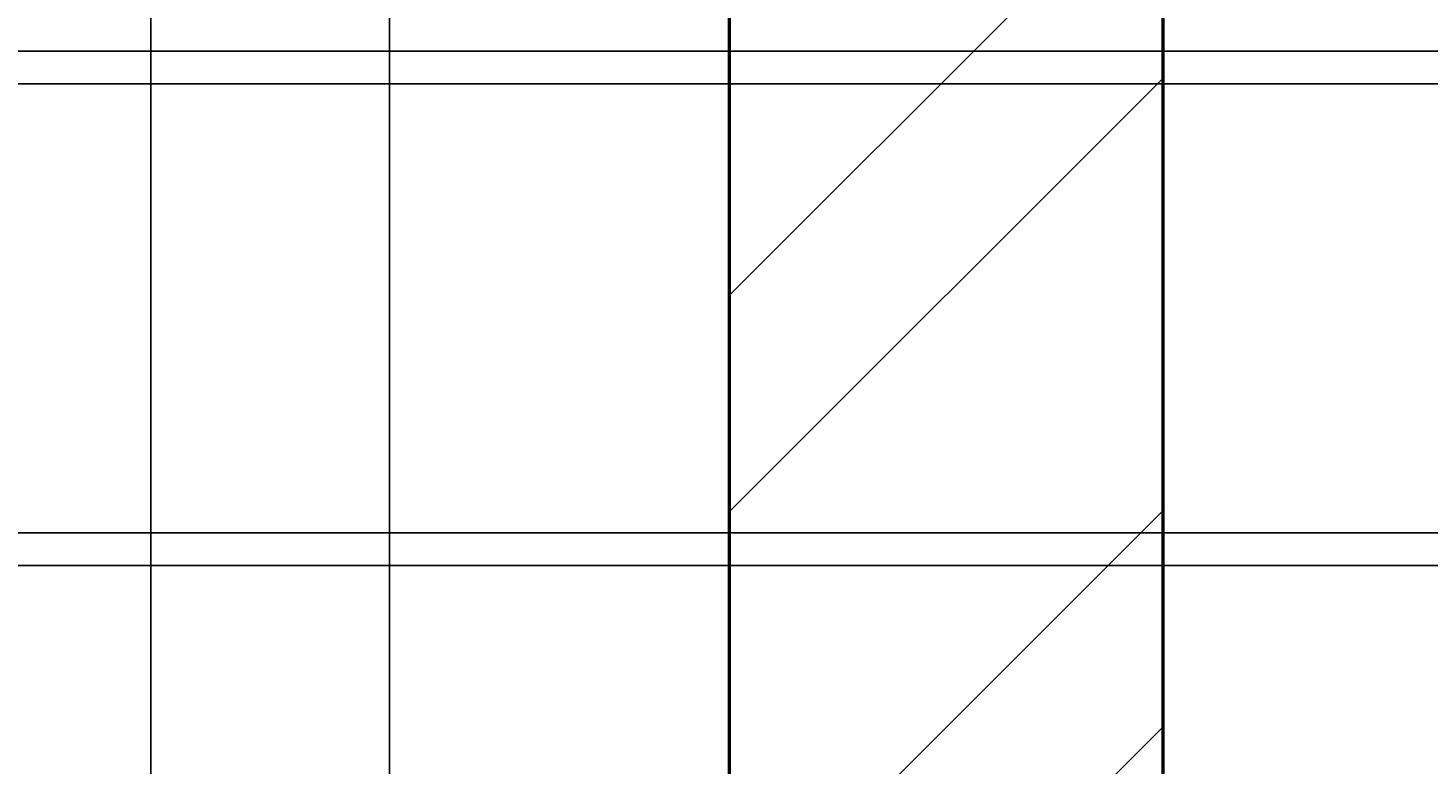
# Model space of a CAD drawing. Units: inches. Extents: x 2812 to 3051, y 1398 to 1659.
# Tile 35 of 65: x 3004 to 3033, y 1433 to 1448. Entities that reach past the tile are written whole.
import ezdxf

# ---------------------------------------------------------------- set-up
doc = ezdxf.new("R2010")
doc.units = ezdxf.units.IN
for name, color, linetype, lineweight in [('A-ANNO-DIMS', 2, 'Continuous', 18), ('S-CONC', 7, 'Continuous', 50), ('S-CONC-PATT', 8, 'Continuous', 18)]:
    doc.layers.add(name, color=color, linetype=linetype, lineweight=lineweight)
doc.styles.get("Standard").update_dxf_attribs({"font": 'arial.ttf'})
doc.dimstyles.get("Standard").update_dxf_attribs({"dimtxt": 0.18, "dimasz": 0.18, "dimexe": 0.18, "dimexo": 0.0625, "dimgap": 0.09, "dimtad": 0, "dimtih": 1, "dimtoh": 1, "dimdec": 4, "dimzin": 0, "dimdsep": 46, "dimtxsty": 'Standard', "dimcen": 0.09, "dimadec": 0, "dimazin": 0, "dimtfac": 1, "dimtdec": 4, "dimtofl": 0, "dimtmove": 0, "dimatfit": 3, "dimfxl": 1, "dimtolj": 1, "dimtzin": 0, "dimarcsym": 0})

# ---------------------------------------------------------------- blocks, each defined once
blk = doc.blocks.new('*D33')
at = {"layer": 'A-ANNO-DIMS', "color": 0, "lineweight": -2, "transparency": 16777216}
for p, q in [((3011.337, 1597.982), (3011.337, 1397.505)), ((3018.385, 1559.757), (3018.385, 1397.505)), ((3011.517, 1397.685), (3014.468, 1397.685)), ((3018.205, 1397.685), (3015.254, 1397.685))]:
    blk.add_line(p, q, dxfattribs=at)
at = {"layer": 'A-ANNO-DIMS', "color": 0, "transparency": 16777216}
for points in [[(3011.517, 1397.715), (3011.517, 1397.655), (3011.337, 1397.685)], [(3018.205, 1397.715), (3018.205, 1397.655), (3018.385, 1397.685)]]:
    blk.add_solid(points, dxfattribs=at)
at = {"layer": 'Defpoints', "color": 0, "transparency": 16777216}
for p in [(3011.337, 1598.044), (3018.385, 1559.82), (3018.385, 1397.685)]:
    blk.add_point(p, dxfattribs=at)
at = {"layer": 'A-ANNO-DIMS', "color": 0, "transparency": 16777216, "insert": (3014.861, 1397.685), "char_height": 0.18, "attachment_point": 5}
blk.add_mtext('\\A1;7.048', dxfattribs=at)
blk = doc.blocks.new('*D34')
at = {"layer": 'A-ANNO-DIMS', "color": 0, "lineweight": -2, "transparency": 16777216}
for p, q in [((3038.462, 1593.482), (3038.462, 1397.505)), ((3027.385, 1550.757), (3027.385, 1397.505)), ((3027.565, 1397.685), (3032.468, 1397.685)), ((3038.282, 1397.685), (3033.379, 1397.685))]:
    blk.add_line(p, q, dxfattribs=at)
at = {"layer": 'A-ANNO-DIMS', "color": 0, "transparency": 16777216}
for points in [[(3027.565, 1397.715), (3027.565, 1397.655), (3027.385, 1397.685)], [(3038.282, 1397.715), (3038.282, 1397.655), (3038.462, 1397.685)]]:
    blk.add_solid(points, dxfattribs=at)
at = {"layer": 'Defpoints', "color": 0, "transparency": 16777216}
for p in [(3038.462, 1593.544), (3027.385, 1550.82), (3038.462, 1397.685)]:
    blk.add_point(p, dxfattribs=at)
at = {"layer": 'A-ANNO-DIMS', "color": 0, "transparency": 16777216, "insert": (3032.923, 1397.685), "char_height": 0.18, "attachment_point": 5}
blk.add_mtext('\\A1;11.077', dxfattribs=at)
blk = doc.blocks.new('*D47')
at = {"layer": 'A-ANNO-DIMS', "color": 0, "lineweight": -2, "transparency": 16777216}
for p, q in [((2970.385, 1487.973), (2970.385, 1397.505)), ((3006.385, 1487.973), (3006.385, 1397.505)), ((2970.565, 1397.685), (2988.166, 1397.685)), ((3006.205, 1397.685), (2988.604, 1397.685))]:
    blk.add_line(p, q, dxfattribs=at)
at = {"layer": 'A-ANNO-DIMS', "color": 0, "transparency": 16777216}
for points in [[(2970.565, 1397.715), (2970.565, 1397.655), (2970.385, 1397.685)], [(3006.205, 1397.715), (3006.205, 1397.655), (3006.385, 1397.685)]]:
    blk.add_solid(points, dxfattribs=at)
at = {"layer": 'Defpoints', "color": 0, "transparency": 16777216}
for p in [(2970.385, 1488.035), (3006.385, 1488.035), (3006.385, 1397.685)]:
    blk.add_point(p, dxfattribs=at)
at = {"layer": 'A-ANNO-DIMS', "color": 0, "transparency": 16777216, "insert": (2988.385, 1397.685), "char_height": 0.18, "attachment_point": 5}
blk.add_mtext('\\A1;36', dxfattribs=at)
blk = doc.blocks.new('*D48')
at = {"layer": 'A-ANNO-DIMS', "color": 0, "lineweight": -2, "transparency": 16777216}
for p, q in [((3006.385, 1487.973), (3006.385, 1397.505)), ((3036.385, 1409.973), (3036.385, 1397.505)), ((3006.565, 1397.685), (3021.166, 1397.685)), ((3036.205, 1397.685), (3021.603, 1397.685))]:
    blk.add_line(p, q, dxfattribs=at)
at = {"layer": 'A-ANNO-DIMS', "color": 0, "transparency": 16777216}
for points in [[(3006.565, 1397.715), (3006.565, 1397.655), (3006.385, 1397.685)], [(3036.205, 1397.715), (3036.205, 1397.655), (3036.385, 1397.685)]]:
    blk.add_solid(points, dxfattribs=at)
at = {"layer": 'Defpoints', "color": 0, "transparency": 16777216}
for p in [(3006.385, 1488.035), (3036.385, 1410.035), (3036.385, 1397.685)]:
    blk.add_point(p, dxfattribs=at)
at = {"layer": 'A-ANNO-DIMS', "color": 0, "transparency": 16777216, "insert": (3021.385, 1397.685), "char_height": 0.18, "attachment_point": 5}
blk.add_mtext('\\A1;30', dxfattribs=at)
blk = doc.blocks.new('*D65')
at = {"layer": 'A-ANNO-DIMS', "color": 0, "lineweight": -2, "transparency": 16777216}
for p, q in [((2920.62, 1437.426), (3051.178, 1437.426)), ((3050.998, 1437.246), (3050.998, 1432.608)), ((3050.998, 1427.606), (3050.998, 1432.245)), ((2929.438, 1427.426), (3051.178, 1427.426))]:
    blk.add_line(p, q, dxfattribs=at)
at = {"layer": 'A-ANNO-DIMS', "color": 0, "transparency": 16777216}
for points in [[(3050.968, 1437.246), (3051.028, 1437.246), (3050.998, 1437.426)], [(3050.968, 1427.606), (3051.028, 1427.606), (3050.998, 1427.426)]]:
    blk.add_solid(points, dxfattribs=at)
at = {"layer": 'Defpoints', "color": 0, "transparency": 16777216}
for p in [(2920.558, 1437.426), (3050.998, 1437.426), (2929.375, 1427.426)]:
    blk.add_point(p, dxfattribs=at)
at = {"layer": 'A-ANNO-DIMS', "color": 0, "transparency": 16777216, "insert": (3050.998, 1432.426), "char_height": 0.18, "attachment_point": 5}
blk.add_mtext('\\A1;10', dxfattribs=at)
blk = doc.blocks.new('*D66')
at = {"layer": 'A-ANNO-DIMS', "color": 0, "lineweight": -2, "transparency": 16777216}
for p, q in [((2914.018, 1447.426), (3051.178, 1447.426)), ((3050.998, 1447.246), (3050.998, 1442.608)), ((3050.998, 1437.606), (3050.998, 1442.245)), ((2920.62, 1437.426), (3051.178, 1437.426))]:
    blk.add_line(p, q, dxfattribs=at)
at = {"layer": 'A-ANNO-DIMS', "color": 0, "transparency": 16777216}
for points in [[(3050.968, 1447.246), (3051.028, 1447.246), (3050.998, 1447.426)], [(3050.968, 1437.606), (3051.028, 1437.606), (3050.998, 1437.426)]]:
    blk.add_solid(points, dxfattribs=at)
at = {"layer": 'Defpoints', "color": 0, "transparency": 16777216}
for p in [(2913.955, 1447.426), (3050.998, 1447.426), (2920.558, 1437.426)]:
    blk.add_point(p, dxfattribs=at)
at = {"layer": 'A-ANNO-DIMS', "color": 0, "transparency": 16777216, "insert": (3050.998, 1442.426), "char_height": 0.18, "attachment_point": 5}
blk.add_mtext('\\A1;10', dxfattribs=at)
blk = doc.blocks.new('*D67')
at = {"layer": 'A-ANNO-DIMS', "color": 0, "lineweight": -2, "transparency": 16777216}
for p, q in [((2906.065, 1457.426), (3051.178, 1457.426)), ((3050.998, 1457.246), (3050.998, 1452.608)), ((3050.998, 1447.606), (3050.998, 1452.245)), ((2914.018, 1447.426), (3051.178, 1447.426))]:
    blk.add_line(p, q, dxfattribs=at)
at = {"layer": 'A-ANNO-DIMS', "color": 0, "transparency": 16777216}
for points in [[(3050.968, 1457.246), (3051.028, 1457.246), (3050.998, 1457.426)], [(3050.968, 1447.606), (3051.028, 1447.606), (3050.998, 1447.426)]]:
    blk.add_solid(points, dxfattribs=at)
at = {"layer": 'Defpoints', "color": 0, "transparency": 16777216}
for p in [(2906.002, 1457.426), (3050.998, 1457.426), (2913.955, 1447.426)]:
    blk.add_point(p, dxfattribs=at)
at = {"layer": 'A-ANNO-DIMS', "color": 0, "transparency": 16777216, "insert": (3050.998, 1452.426), "char_height": 0.18, "attachment_point": 5}
blk.add_mtext('\\A1;10', dxfattribs=at)
blk = doc.blocks.new('*D79')
at = {"layer": 'A-ANNO-DIMS', "color": 0, "lineweight": -2, "transparency": 16777216}
for p, q in [((3003.284, 1436.747), (3051.178, 1436.747)), ((3050.998, 1436.567), (3050.998, 1431.929)), ((3050.998, 1426.927), (3050.998, 1431.565)), ((3012.899, 1426.747), (3051.178, 1426.747))]:
    blk.add_line(p, q, dxfattribs=at)
at = {"layer": 'A-ANNO-DIMS', "color": 0, "transparency": 16777216}
for points in [[(3050.968, 1436.567), (3051.028, 1436.567), (3050.998, 1436.747)], [(3050.968, 1426.927), (3051.028, 1426.927), (3050.998, 1426.747)]]:
    blk.add_solid(points, dxfattribs=at)
at = {"layer": 'Defpoints', "color": 0, "transparency": 16777216}
for p in [(3003.221, 1436.747), (3050.998, 1436.747), (3012.837, 1426.747)]:
    blk.add_point(p, dxfattribs=at)
at = {"layer": 'A-ANNO-DIMS', "color": 0, "transparency": 16777216, "insert": (3050.998, 1431.747), "char_height": 0.18, "attachment_point": 5}
blk.add_mtext('\\A1;10', dxfattribs=at)
blk = doc.blocks.new('*D80')
at = {"layer": 'A-ANNO-DIMS', "color": 0, "lineweight": -2, "transparency": 16777216}
for p, q in [((2996.018, 1446.747), (3051.178, 1446.747)), ((3050.998, 1446.567), (3050.998, 1441.929)), ((3050.998, 1436.927), (3050.998, 1441.565)), ((3003.284, 1436.747), (3051.178, 1436.747))]:
    blk.add_line(p, q, dxfattribs=at)
at = {"layer": 'A-ANNO-DIMS', "color": 0, "transparency": 16777216}
for points in [[(3050.968, 1446.567), (3051.028, 1446.567), (3050.998, 1446.747)], [(3050.968, 1436.927), (3051.028, 1436.927), (3050.998, 1436.747)]]:
    blk.add_solid(points, dxfattribs=at)
at = {"layer": 'Defpoints', "color": 0, "transparency": 16777216}
for p in [(2995.956, 1446.747), (3050.998, 1446.747), (3003.221, 1436.747)]:
    blk.add_point(p, dxfattribs=at)
at = {"layer": 'A-ANNO-DIMS', "color": 0, "transparency": 16777216, "insert": (3050.998, 1441.747), "char_height": 0.18, "attachment_point": 5}
blk.add_mtext('\\A1;10', dxfattribs=at)
blk = doc.blocks.new('*D81')
at = {"layer": 'A-ANNO-DIMS', "color": 0, "lineweight": -2, "transparency": 16777216}
for p, q in [((2988.31, 1456.747), (3051.178, 1456.747)), ((3050.998, 1456.567), (3050.998, 1451.929)), ((3050.998, 1446.927), (3050.998, 1451.565)), ((2996.018, 1446.747), (3051.178, 1446.747))]:
    blk.add_line(p, q, dxfattribs=at)
at = {"layer": 'A-ANNO-DIMS', "color": 0, "transparency": 16777216}
for points in [[(3050.968, 1456.567), (3051.028, 1456.567), (3050.998, 1456.747)], [(3050.968, 1446.927), (3051.028, 1446.927), (3050.998, 1446.747)]]:
    blk.add_solid(points, dxfattribs=at)
at = {"layer": 'Defpoints', "color": 0, "transparency": 16777216}
for p in [(2988.248, 1456.747), (3050.998, 1456.747), (2995.956, 1446.747)]:
    blk.add_point(p, dxfattribs=at)
at = {"layer": 'A-ANNO-DIMS', "color": 0, "transparency": 16777216, "insert": (3050.998, 1451.747), "char_height": 0.18, "attachment_point": 5}
blk.add_mtext('\\A1;10', dxfattribs=at)

msp = doc.modelspace()

# ---------------------------------------------------------------- hatches: boundary and pattern name
at = {"layer": 'S-CONC-PATT'}
h = msp.add_hatch(dxfattribs=at)
h.set_pattern_fill('ANSI32', color=256)
h.paths.add_polyline_path([(3027.3849, 1646.82), (2835.3849, 1646.82), (2835.3849, 1603.2296), (2844.3849, 1603.2296), (2844.3849, 1637.82), (3018.3849, 1637.82), (3018.3849, 1602.5441), (3027.3849, 1602.5441)])
h.paths.add_polyline_path([(2844.3849, 1594.2296), (2835.3849, 1594.2296), (2835.3849, 1550.82), (3027.3849, 1550.82), (3027.3849, 1593.5441), (3018.3849, 1593.5441), (3018.3849, 1559.82), (2844.3849, 1559.82)])
h.paths.add_polyline_path([(2844.3849, 1482.0354), (2835.3849, 1482.0354), (2835.3849, 1463.4959), (2844.3849, 1463.4959)])
h.paths.add_polyline_path([(2844.3849, 1461.4959), (2835.3849, 1461.4959), (2835.3849, 1416.0354), (2844.3849, 1416.0354)])
h.paths.add_polyline_path([(3027.3849, 1482.0354), (3018.3849, 1482.0354), (3018.3849, 1463.2854), (3027.3849, 1463.2854)])
h.paths.add_polyline_path([(3027.3849, 1461.2854), (3018.3849, 1461.2854), (3018.3849, 1416.0354), (3027.3849, 1416.0354)])
h.paths.add_polyline_path([(2961.3849, 1448.4738), (2952.3849, 1448.4738), (2952.3849, 1416.0354), (2961.3849, 1416.0354)])
h.paths.add_polyline_path([(2961.3849, 1462.3026), (2952.3849, 1462.3026), (2952.3849, 1450.4738), (2961.3849, 1450.4738)])
h.paths.add_polyline_path([(2961.3849, 1472.0354), (2952.3849, 1472.0354), (2952.3849, 1462.3026), (2961.3849, 1462.3026)])

# ---------------------------------------------------------------- linework, layer by layer
at = {"layer": 'S-CONC'}
for p, q in [((3018.3849, 1482.0354), (3018.3849, 1416.0354)), ((3027.3849, 1482.0354), (3027.3849, 1416.0354))]:
    msp.add_line(p, q, dxfattribs=at)

# ---------------------------------------------------------------- dimensions: what is measured, and where the dimension line sits
at = {"layer": 'A-ANNO-DIMS'}
for base, p1, p2, override, picture, middle in [((3018.3849, 1397.6854), (3011.3373, 1598.0441), (3018.3849, 1559.82), {"dimdec": 3, "dimlfac": 1, "dimrnd": 0, "dimzin": 0, "dimdsep": 46, "dimlunit": 2}, '*D33', (3014.8611, 1397.6854)), ((3038.4621, 1397.6854), (3027.3849, 1550.82), (3038.4621, 1593.5441), {"dimdec": 3, "dimlfac": 1, "dimrnd": 0, "dimzin": 0, "dimdsep": 46, "dimlunit": 2}, '*D34', (3032.9235, 1397.6854)), ((3006.3849, 1397.6854), (2970.3849, 1488.0354), (3006.3849, 1488.0354), {"dimdec": 0, "dimlfac": 1, "dimrnd": 0, "dimzin": 0, "dimdsep": 46, "dimlunit": 2}, '*D47', (2988.3849, 1397.6854)), ((3036.3849, 1397.6854), (3006.3849, 1488.0354), (3036.3849, 1410.0354), {"dimdec": 0, "dimlfac": 1, "dimrnd": 0, "dimzin": 0, "dimdsep": 46, "dimlunit": 2}, '*D48', (3021.3849, 1397.6854))]:
    dim = msp.add_linear_dim(base=base, p1=p1, p2=p2, dimstyle='Standard', override=override, dxfattribs=at)
    dim.commit()
    dim.dimension.update_dxf_attribs({"geometry": picture, "text_midpoint": middle})
for base, p1, p2, picture, middle in [((3050.998, 1457.4265), (2913.9551, 1447.4265), (2906.0021, 1457.4265), '*D67', (3050.998, 1452.4265)), ((3050.998, 1456.7474), (2995.9558, 1446.7474), (2988.2478, 1456.7474), '*D81', (3050.998, 1451.7474)), ((3050.998, 1447.4265), (2920.5577, 1437.4265), (2913.9551, 1447.4265), '*D66', (3050.998, 1442.4265)), ((3050.998, 1446.7474), (3003.2213, 1436.7474), (2995.9558, 1446.7474), '*D80', (3050.998, 1441.7474)), ((3050.998, 1437.4265), (2929.3751, 1427.4265), (2920.5577, 1437.4265), '*D65', (3050.998, 1432.4265)), ((3050.998, 1436.7474), (3012.8368, 1426.7474), (3003.2213, 1436.7474), '*D79', (3050.998, 1431.7474))]:
    dim = msp.add_linear_dim(base=base, p1=p1, p2=p2, angle=90, dimstyle='Standard', override={"dimdec": 0, "dimlfac": 1, "dimrnd": 0, "dimzin": 0, "dimdsep": 46, "dimlunit": 2}, dxfattribs=at)
    dim.commit()
    dim.dimension.update_dxf_attribs({"geometry": picture, "text_midpoint": middle})

doc.saveas('drawing.dxf')
